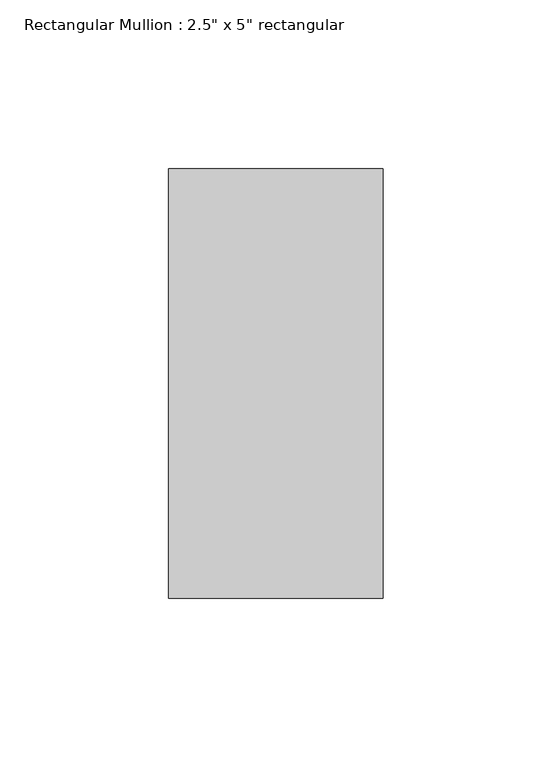
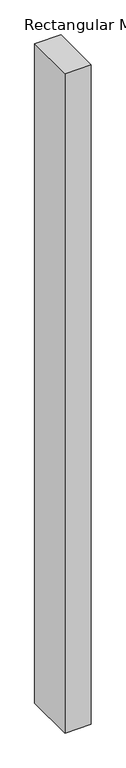
"""IFC4 building model written with IfcOpenShell, lengths in millimetres: member geometry."""

from ifc_helpers import new_model, si_unit, frame, origin, place, context, project, spatial, polyline, outline, extrude, source, transform, mapped, element, save


def member_cf2a6f2c(model_context):
    return source(origin(), model_context, "Body", "SweptSolid", [
        extrude(outline(polyline([(31.75, 63.5), (31.75, -63.5), (-31.75, -63.5), (-31.75, 63.5), (31.75, 63.5)])), frame((0.0, 0.0, -1696.2528693), z_axis=(0.0, 0.0, 1.0), x_axis=(1.0, 0.0, 0.0)), (0.0, 0.0, 1.0), 1696.2528693),
    ])


if __name__ == "__main__":
    model = new_model("IFC4")
    model_context = context("Model", 3, world=origin())
    ifc_project = project(units=[si_unit("LENGTHUNIT", "METRE", prefix="MILLI")], contexts=[model_context])
    site = spatial("IfcSite", under=ifc_project)
    building = spatial("IfcBuilding", under=site)
    placement = place(None, origin())
    member_shape = member_cf2a6f2c(model_context)
    element("IfcMember", 1, ObjectType="Rectangular Mullion : 2.5\" x 5\" rectangular", at=placement, inside=building, context=model_context, shape_type="MappedRepresentation", body=[
        mapped(member_shape, transform((0.0, 0.0, 0.0), x_axis=(1.0, 0.0, 0.0), y_axis=(0.0, 1.0, 0.0), z_axis=(0.0, 0.0, 1.0))),
    ])
    save(model, "model.ifc")

# Revit data of these elements
# Type "Rectangular Mullion : 2.5\" x 5\" rectangular"
#   built-in parameter 1007304 = 0.416667 (stored number, unit not read)
#   built-in parameter 1007301 = 0.104167 (stored number, unit not read)
#   built-in parameter 1007300 = 0.104167 (stored number, unit not read)
# Element 1 (IfcMember, "Rectangular Mullion : 2.5\" x 5\" rectangular")
#   Materials on its faces: "Aluminum"
# Materials
#   "Aluminum": class "Metal", colour RGB 247 247 247, transparency 0, Description = "Aluminum 6061", Cost = 0
